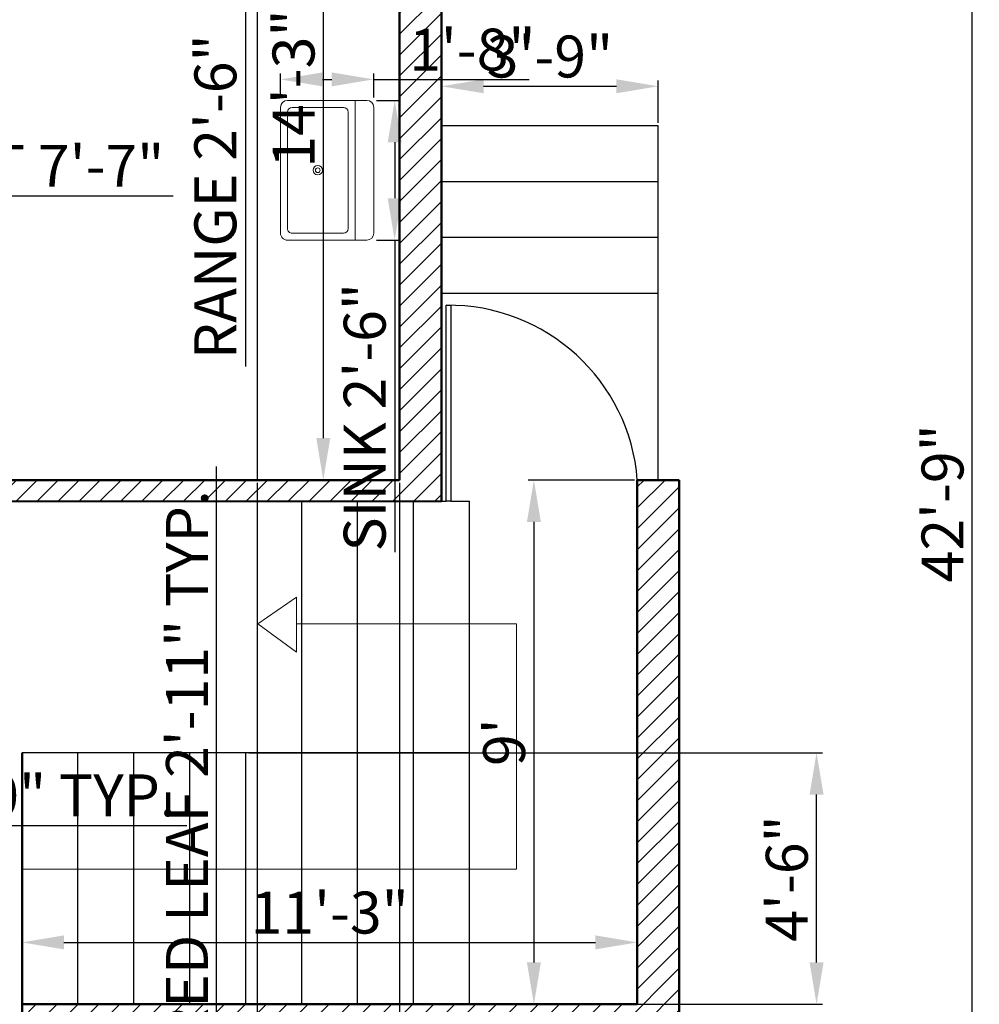
# Model space of a CAD drawing. Units: inches. Extents: x 5928 to 6612, y 5674 to 6320.
# Tile 4 of 5: x 6407 to 6612, y 5862 to 6074. Entities that reach past the tile are written whole.
import ezdxf

# ---------------------------------------------------------------- set-up
doc = ezdxf.new("R2010")
doc.units = ezdxf.units.IN
for name, color, linetype, lineweight in [('A-ANNO-DIMS', 2, 'Continuous', 18), ('A-ANNO-SYMB', 2, 'Continuous', 18), ('A-DOOR', 3, 'Continuous', 25), ('A-FLOR-CASE', 8, 'Continuous', 25), ('A-FLOR-FIXT', 9, 'Continuous', 18), ('A-FLOR-STRS', 7, 'Continuous', 25), ('A-WALL', 7, 'Continuous', 50), ('A-WALL-PATT', 252, 'Continuous', 13)]:
    doc.layers.add(name, color=color, linetype=linetype, lineweight=lineweight)
doc.styles.get("Standard").update_dxf_attribs({"font": 'arial.ttf'})
doc.dimstyles.new('ISO-25', dxfattribs={"dimtxt": 9, "dimasz": 9, "dimexe": 1.25, "dimexo": 0.625, "dimtad": 1, "dimdec": 1, "dimrnd": 9, "dimlunit": 3, "dimtxsty": 'Standard', "dimcen": 2.5, "dimadec": 0, "dimazin": 0, "dimtfac": 1, "dimtdec": 1, "dimtmove": 0, "dimatfit": 3, "dimfxl": 1, "dimarcsym": 0})

# ---------------------------------------------------------------- blocks, each defined once
blk = doc.blocks.new('*D1')
at = {"layer": 'A-ANNO-DIMS', "color": 0, "lineweight": -2, "transparency": 16777216}
for p, q in [((6497.03, 6051.41), (6497.03, 6060.5)), ((6543.53, 6051.41), (6543.53, 6060.5)), ((6506.03, 6059.25), (6534.53, 6059.25))]:
    blk.add_line(p, q, dxfattribs=at)
at = {"layer": 'A-ANNO-DIMS', "color": 0, "transparency": 16777216}
for points in [[(6506.03, 6060.75), (6506.03, 6057.75), (6497.03, 6059.25)], [(6534.53, 6060.75), (6534.53, 6057.75), (6543.53, 6059.25)]]:
    blk.add_solid(points, dxfattribs=at)
at = {"layer": 'Defpoints', "color": 0, "transparency": 16777216}
for p in [(6543.53, 6059.25), (6497.03, 6050.78), (6543.53, 6050.78)]:
    blk.add_point(p, dxfattribs=at)
at = {"layer": 'A-ANNO-DIMS', "color": 0, "transparency": 16777216, "insert": (6520.28, 6064.47), "char_height": 9, "attachment_point": 5}
blk.add_mtext('3\'-9"', dxfattribs=at)
blk = doc.blocks.new('Sink-single - 30 in top')
blk.add_line((-15, -3.999996), (15, -3.999996))
for points in [[(-13.5, 0), (13.5, 0)], [(-15, -18.499996), (-15, -1.5)], [(15, -1.5), (15, -18.499996)], [(-12.5, -5.499996), (12.5, -5.499996)], [(-13.5, -17.499996), (-13.5, -6.499996)], [(13.5, -6.499996), (13.5, -17.499996)], [(12.5, -18.499996), (-12.5, -18.499996)], [(13.5, -19.999996), (-13.5, -19.999996)]]:
    blk.add_lwpolyline(points)
for radius in [1, 0.5]:
    blk.add_circle((0, -11.999996), radius)
for centre, radius, start, end in [((-13.5, -1.5), 1.5, 90, 180), ((13.5, -1.5), 1.5, 0, 90), ((-12.5, -6.499996), 1, 90, 180), ((12.5, -6.499996), 1, 0, 90), ((-13.5, -18.499996), 1.5, 180, 270), ((-12.5, -17.499996), 1, 180, 270), ((12.5, -17.499996), 1, 270, 0), ((13.5, -18.499996), 1.5, 270, 0)]:
    blk.add_arc(centre, radius, start, end)
blk = doc.blocks.new('*D32')
at = {"layer": 'A-ANNO-DIMS', "color": 0, "lineweight": -2, "transparency": 16777216}
for p, q in [((6538.4, 5974.76), (6515.59, 5974.76)), ((6516.84, 5965.76), (6516.84, 5871.26)), ((6538.4, 5862.26), (6515.59, 5862.26))]:
    blk.add_line(p, q, dxfattribs=at)
at = {"layer": 'A-ANNO-DIMS', "color": 0, "transparency": 16777216}
for points in [[(6515.34, 5965.76), (6518.34, 5965.76), (6516.84, 5974.76)], [(6515.34, 5871.26), (6518.34, 5871.26), (6516.84, 5862.26)]]:
    blk.add_solid(points, dxfattribs=at)
at = {"layer": 'Defpoints', "color": 0, "transparency": 16777216}
for p in [(6539.03, 5974.76), (6516.84, 5862.26), (6539.03, 5862.26)]:
    blk.add_point(p, dxfattribs=at)
at = {"layer": 'A-ANNO-DIMS', "color": 0, "transparency": 16777216, "insert": (6511.62, 5918.51), "char_height": 9, "attachment_point": 5, "rotation": 90}
blk.add_mtext("9'", dxfattribs=at)
blk = doc.blocks.new('*D33')
at = {"layer": 'A-ANNO-DIMS', "color": 0, "lineweight": -2, "transparency": 16777216}
for p, q in [((6407.03, 5862.89), (6407.03, 5876.8)), ((6539.03, 5862.89), (6539.03, 5876.8)), ((6416.03, 5875.55), (6530.03, 5875.55))]:
    blk.add_line(p, q, dxfattribs=at)
at = {"layer": 'A-ANNO-DIMS', "color": 0, "transparency": 16777216}
for points in [[(6416.03, 5877.05), (6416.03, 5874.05), (6407.03, 5875.55)], [(6530.03, 5877.05), (6530.03, 5874.05), (6539.03, 5875.55)]]:
    blk.add_solid(points, dxfattribs=at)
at = {"layer": 'Defpoints', "color": 0, "transparency": 16777216}
for p in [(6539.03, 5875.55), (6407.03, 5862.26), (6539.03, 5862.26)]:
    blk.add_point(p, dxfattribs=at)
at = {"layer": 'A-ANNO-DIMS', "color": 0, "transparency": 16777216, "insert": (6473.03, 5880.78), "char_height": 9, "attachment_point": 5}
blk.add_mtext('11\'-3"', dxfattribs=at)
blk = doc.blocks.new('*D34')
at = {"layer": 'A-ANNO-DIMS', "color": 0, "lineweight": -2, "transparency": 16777216}
for p, q in [((6487.4, 6142.76), (6470.41, 6142.76)), ((6471.66, 6133.76), (6471.66, 5983.76)), ((6487.4, 5974.76), (6470.41, 5974.76))]:
    blk.add_line(p, q, dxfattribs=at)
at = {"layer": 'A-ANNO-DIMS', "color": 0, "transparency": 16777216}
for points in [[(6470.16, 6133.76), (6473.16, 6133.76), (6471.66, 6142.76)], [(6470.16, 5983.76), (6473.16, 5983.76), (6471.66, 5974.76)]]:
    blk.add_solid(points, dxfattribs=at)
at = {"layer": 'Defpoints', "color": 0, "transparency": 16777216}
for p in [(6488.03, 6142.76), (6471.66, 5974.76), (6488.03, 5974.76)]:
    blk.add_point(p, dxfattribs=at)
at = {"layer": 'A-ANNO-DIMS', "color": 0, "transparency": 16777216, "insert": (6466.44, 6058.76), "char_height": 9, "attachment_point": 5, "rotation": 90}
blk.add_mtext('14\'-3"', dxfattribs=at)
blk = doc.blocks.new('*D37')
at = {"layer": 'A-ANNO-DIMS', "color": 0, "lineweight": -2, "transparency": 16777216}
for p, q in [((6497.65, 6228.26), (6612.14, 6228.26)), ((6610.89, 5720.26), (6610.89, 6219.26)), ((6424.38, 5711.26), (6612.14, 5711.26))]:
    blk.add_line(p, q, dxfattribs=at)
at = {"layer": 'A-ANNO-DIMS', "color": 0, "transparency": 16777216}
for points in [[(6609.39, 6219.26), (6612.39, 6219.26), (6610.89, 6228.26)], [(6609.39, 5720.26), (6612.39, 5720.26), (6610.89, 5711.26)]]:
    blk.add_solid(points, dxfattribs=at)
at = {"layer": 'Defpoints', "color": 0, "transparency": 16777216}
for p in [(6497.03, 6228.26), (6610.89, 6228.26), (6423.76, 5711.26)]:
    blk.add_point(p, dxfattribs=at)
at = {"layer": 'A-ANNO-DIMS', "color": 0, "transparency": 16777216, "insert": (6605.67, 5969.76), "char_height": 9, "attachment_point": 5, "rotation": 90}
blk.add_mtext('42\'-9"', dxfattribs=at)
blk = doc.blocks.new('DOOR-LEAF-42IN')
for p, q in [((0, 0), (0, 42)), ((0, 42), (1, 42)), ((1, 42), (1, 0)), ((-1, 0), (0, 0)), ((1, 0), (0, 0))]:
    blk.add_line(p, q)
blk = doc.blocks.new('*D56')
at = {"layer": 'A-ANNO-DIMS', "color": 0, "lineweight": -2, "transparency": 16777216}
for p, q in [((6280.02, 5909.02), (6280.02, 5899.4)), ((6340.02, 5909.02), (6340.02, 5899.4)), ((6289.02, 5900.65), (6331.02, 5900.65)), ((6340.02, 5900.65), (6442.41, 5900.65))]:
    blk.add_line(p, q, dxfattribs=at)
at = {"layer": 'A-ANNO-DIMS', "color": 0, "transparency": 16777216}
for points in [[(6289.02, 5902.15), (6289.02, 5899.15), (6280.02, 5900.65)], [(6331.02, 5902.15), (6331.02, 5899.15), (6340.02, 5900.65)]]:
    blk.add_solid(points, dxfattribs=at)
at = {"layer": 'Defpoints', "color": 0, "transparency": 16777216}
for p in [(6280.02, 5909.65), (6340.02, 5909.65), (6340.02, 5900.65)]:
    blk.add_point(p, dxfattribs=at)
at = {"layer": 'A-ANNO-DIMS', "color": 0, "transparency": 16777216, "insert": (6395.71, 5905.93), "char_height": 9, "attachment_point": 5}
blk.add_mtext('DESK 5\'-0" TYP.', dxfattribs=at)
blk = doc.blocks.new('*D62')
at = {"layer": 'A-ANNO-DIMS', "color": 0, "lineweight": -2, "transparency": 16777216}
for p, q in [((6448.73, 5820.79), (6448.73, 5977.68)), ((6444.07, 5820.79), (6449.98, 5820.79)), ((6448.73, 5794.57), (6448.73, 5811.79)), ((6444.07, 5785.57), (6449.98, 5785.57))]:
    blk.add_line(p, q, dxfattribs=at)
at = {"layer": 'A-ANNO-DIMS', "color": 0, "transparency": 16777216}
for points in [[(6447.23, 5811.79), (6450.23, 5811.79), (6448.73, 5820.79)], [(6447.23, 5794.57), (6450.23, 5794.57), (6448.73, 5785.57)]]:
    blk.add_solid(points, dxfattribs=at)
at = {"layer": 'Defpoints', "color": 0, "transparency": 16777216}
for p in [(6443.45, 5820.79), (6448.73, 5820.79), (6443.45, 5785.57)]:
    blk.add_point(p, dxfattribs=at)
at = {"layer": 'A-ANNO-DIMS', "color": 0, "transparency": 16777216, "insert": (6443.58, 5903.73), "char_height": 9, "attachment_point": 5, "rotation": 90}
blk.add_mtext('PAIRED LEAF 2\'-11" TYP.', dxfattribs=at)
blk = doc.blocks.new('*D64')
at = {"layer": 'A-ANNO-DIMS', "color": 0, "lineweight": -2, "transparency": 16777216}
for p, q in [((6239.27, 6048.77), (6239.27, 6034.49)), ((6330.27, 6048.77), (6330.27, 6034.49)), ((6248.27, 6035.74), (6321.27, 6035.74)), ((6330.27, 6035.74), (6439.44, 6035.74))]:
    blk.add_line(p, q, dxfattribs=at)
at = {"layer": 'A-ANNO-DIMS', "color": 0, "transparency": 16777216}
for points in [[(6248.27, 6037.24), (6248.27, 6034.24), (6239.27, 6035.74)], [(6321.27, 6037.24), (6321.27, 6034.24), (6330.27, 6035.74)]]:
    blk.add_solid(points, dxfattribs=at)
at = {"layer": 'Defpoints', "color": 0, "transparency": 16777216}
for p in [(6239.27, 6049.39), (6330.27, 6049.39), (6330.27, 6035.74)]:
    blk.add_point(p, dxfattribs=at)
at = {"layer": 'A-ANNO-DIMS', "color": 0, "transparency": 16777216, "insert": (6389.36, 6041.02), "char_height": 9, "attachment_point": 5}
blk.add_mtext('DINING SET 7\'-7"', dxfattribs=at)
blk = doc.blocks.new('*D66')
at = {"layer": 'A-ANNO-DIMS', "color": 0, "lineweight": -2, "transparency": 16777216}
for p, q in [((6458.82, 6111), (6453.69, 6111)), ((6454.94, 6102), (6454.94, 6090)), ((6458.82, 6081), (6453.69, 6081)), ((6454.94, 6081), (6454.94, 5999.09))]:
    blk.add_line(p, q, dxfattribs=at)
at = {"layer": 'A-ANNO-DIMS', "color": 0, "transparency": 16777216}
for points in [[(6453.44, 6102), (6456.44, 6102), (6454.94, 6111)], [(6453.44, 6090), (6456.44, 6090), (6454.94, 6081)]]:
    blk.add_solid(points, dxfattribs=at)
at = {"layer": 'Defpoints', "color": 0, "transparency": 16777216}
for p in [(6459.44, 6111), (6454.94, 6081), (6459.44, 6081)]:
    blk.add_point(p, dxfattribs=at)
at = {"layer": 'A-ANNO-DIMS', "color": 0, "transparency": 16777216, "insert": (6449.67, 6035.54), "char_height": 9, "attachment_point": 5, "rotation": 90}
blk.add_mtext('RANGE 2\'-6"', dxfattribs=at)
blk = doc.blocks.new('*D68')
at = {"layer": 'A-ANNO-DIMS', "color": 0, "lineweight": -2, "transparency": 16777216}
for p, q in [((6483.1, 6056.23), (6488.23, 6056.23)), ((6486.98, 6047.23), (6486.98, 6035.23)), ((6483.1, 6026.23), (6488.23, 6026.23)), ((6486.98, 6026.23), (6486.98, 5959.26))]:
    blk.add_line(p, q, dxfattribs=at)
at = {"layer": 'A-ANNO-DIMS', "color": 0, "transparency": 16777216}
for points in [[(6485.48, 6047.23), (6488.48, 6047.23), (6486.98, 6056.23)], [(6485.48, 6035.23), (6488.48, 6035.23), (6486.98, 6026.23)]]:
    blk.add_solid(points, dxfattribs=at)
at = {"layer": 'Defpoints', "color": 0, "transparency": 16777216}
for p in [(6482.48, 6056.23), (6482.48, 6026.23), (6486.98, 6026.23)]:
    blk.add_point(p, dxfattribs=at)
at = {"layer": 'A-ANNO-DIMS', "color": 0, "transparency": 16777216, "insert": (6481.7, 5988.24), "char_height": 9, "attachment_point": 5, "rotation": 90}
blk.add_mtext('SINK 2\'-6"', dxfattribs=at)
blk = doc.blocks.new('*D69')
at = {"layer": 'A-ANNO-DIMS', "color": 0, "lineweight": -2, "transparency": 16777216}
for p, q in [((6462.48, 6056.85), (6462.48, 6061.98)), ((6482.48, 6056.85), (6482.48, 6061.98)), ((6471.48, 6060.73), (6473.48, 6060.73)), ((6482.48, 6060.73), (6515.81, 6060.73))]:
    blk.add_line(p, q, dxfattribs=at)
at = {"layer": 'A-ANNO-DIMS', "color": 0, "transparency": 16777216}
for points in [[(6471.48, 6062.23), (6471.48, 6059.23), (6462.48, 6060.73)], [(6473.48, 6062.23), (6473.48, 6059.23), (6482.48, 6060.73)]]:
    blk.add_solid(points, dxfattribs=at)
at = {"layer": 'Defpoints', "color": 0, "transparency": 16777216}
for p in [(6482.48, 6060.73), (6462.48, 6056.23), (6482.48, 6056.23)]:
    blk.add_point(p, dxfattribs=at)
at = {"layer": 'A-ANNO-DIMS', "color": 0, "transparency": 16777216, "insert": (6503.64, 6065.95), "char_height": 9, "attachment_point": 5}
blk.add_mtext('1\'-8"', dxfattribs=at)
blk = doc.blocks.new('*D77')
at = {"layer": 'A-ANNO-DIMS', "color": 0, "lineweight": -2, "transparency": 16777216}
for p, q in [((6457.49, 5974.14), (6457.49, 5680.56)), ((6488.03, 5974.14), (6488.03, 5680.56)), ((6466.49, 5681.81), (6479.03, 5681.81)), ((6488.03, 5681.81), (6543.33, 5681.81))]:
    blk.add_line(p, q, dxfattribs=at)
at = {"layer": 'A-ANNO-DIMS', "color": 0, "transparency": 16777216}
for points in [[(6466.49, 5683.31), (6466.49, 5680.31), (6457.49, 5681.81)], [(6479.03, 5683.31), (6479.03, 5680.31), (6488.03, 5681.81)]]:
    blk.add_solid(points, dxfattribs=at)
at = {"layer": 'Defpoints', "color": 0, "transparency": 16777216}
for p in [(6457.49, 5974.76), (6488.03, 5974.76), (6488.03, 5681.81)]:
    blk.add_point(p, dxfattribs=at)
at = {"layer": 'A-ANNO-DIMS', "color": 0, "transparency": 16777216, "insert": (6520.18, 5687.09), "char_height": 9, "attachment_point": 5}
blk.add_mtext('2\'-6 1/2"', dxfattribs=at)
blk = doc.blocks.new('*D78')
at = {"layer": 'A-ANNO-DIMS', "color": 0, "lineweight": -2, "transparency": 16777216}
for p, q in [((6455.65, 5916.26), (6578.73, 5916.26)), ((6577.48, 5871.26), (6577.48, 5907.26)), ((6455.65, 5862.26), (6578.73, 5862.26))]:
    blk.add_line(p, q, dxfattribs=at)
at = {"layer": 'A-ANNO-DIMS', "color": 0, "transparency": 16777216}
for points in [[(6575.98, 5907.26), (6578.98, 5907.26), (6577.48, 5916.26)], [(6575.98, 5871.26), (6578.98, 5871.26), (6577.48, 5862.26)]]:
    blk.add_solid(points, dxfattribs=at)
at = {"layer": 'Defpoints', "color": 0, "transparency": 16777216}
for p in [(6455.03, 5916.26), (6577.48, 5916.26), (6455.03, 5862.26)]:
    blk.add_point(p, dxfattribs=at)
at = {"layer": 'A-ANNO-DIMS', "color": 0, "transparency": 16777216, "insert": (6572.26, 5889.26), "char_height": 9, "attachment_point": 5, "rotation": 90}
blk.add_mtext('4\'-6"', dxfattribs=at)

msp = doc.modelspace()

# ---------------------------------------------------------------- hatches: boundary and pattern name
at = {"layer": 'A-WALL-PATT'}
h = msp.add_hatch(dxfattribs=at)
h.set_pattern_fill('ANSI31', color=256)
h.paths.add_polyline_path([(6071.03, 6165.76), (6215.03, 6165.76), (6215.03, 5969.77), (6215.03, 5950.32), (6219.53, 5950.32), (6219.53, 6142.76), (6239.11, 6142.76), (6239.11, 6151.76), (6224.03, 6151.76), (6224.03, 6174.76), (6062.03, 6174.76), (6062.03, 5969.76), (6062.03, 5894.26), (6108.76, 5894.26), (6108.76, 5711.26), (6423.76, 5711.26), (6423.76, 5750.35), (6414.76, 5750.35), (6414.76, 5720.26), (6266.26, 5720.26), (6266.26, 5862.26), (6361.1, 5862.26), (6361.1, 5866.76), (6261.76, 5866.76), (6261.76, 5720.26), (6117.76, 5720.26), (6117.76, 5792.26), (6218.26, 5792.26), (6218.26, 5796.76), (6117.76, 5796.76), (6117.76, 5898.76), (6213.76, 5898.76), (6213.76, 5828.21, -0.018207), (6216.01, 5828.09), (6218.26, 5828.09), (6218.26, 5903.26), (6117.76, 5903.26), (6071.03, 5903.26), (6071.03, 5969.77), (6071.03, 6041.26), (6117.76, 6041.26), (6172.44, 6041.26), (6172.44, 6045.76), (6117.76, 6045.76), (6071.03, 6045.76)])
h.paths.add_polyline_path([(6368.03, 6219.26), (6488.03, 6219.26), (6488.03, 6147.26), (6403.79, 6147.26), (6403.79, 6142.76), (6488.03, 6142.76), (6488.03, 5974.76), (6363.53, 5974.76), (6363.53, 5970.11), (6497.03, 5970.26), (6497.03, 6142.76), (6497.03, 6228.26), (6359.03, 6228.26), (6359.03, 6151.76), (6344.11, 6151.76), (6344.11, 6142.76), (6363.53, 6142.76), (6363.53, 6013.35), (6368.03, 6013.35), (6368.03, 6142.76)])
h.paths.add_polyline_path([(6344.11, 6196.21, 0.265753), (6295.16, 6228.26), (6288.06, 6228.26, 0.265753), (6239.11, 6196.21), (6239.11, 6142.76), (6243.61, 6142.76), (6243.61, 6196.76), (6243.45, 6196.76, -0.514089), (6339.79, 6196.74), (6339.61, 6196.76), (6339.61, 6142.76), (6344.11, 6142.76)])
h.paths.add_polyline_path([(6339.61, 6147.26), (6327.61, 6147.26), (6327.61, 6142.76), (6339.61, 6142.76)], flags=17)
h.paths.add_polyline_path([(6255.61, 6147.26), (6243.61, 6147.26), (6243.61, 6142.76), (6255.61, 6142.76)], flags=17)
h.paths.add_polyline_path([(6548.03, 5974.76), (6539.03, 5974.76), (6539.03, 5862.26), (6407.03, 5862.26), (6407.03, 5853.26), (6414.76, 5853.26), (6414.76, 5820.79), (6423.76, 5820.79), (6423.76, 5853.26), (6548.03, 5853.26)])

# ---------------------------------------------------------------- linework, layer by layer
at = {"layer": 'A-ANNO-SYMB'}
for p, q in [((6457.59, 5943.9), (6465.93, 5949.64)), ((6465.93, 5949.64), (6465.93, 5937.81)), ((6465.93, 5937.81), (6457.59, 5943.9)), ((6513.09, 5943.9), (6465.93, 5943.9)), ((6513.09, 5891.29), (6513.09, 5943.9)), ((6407.03, 5891.29), (6407.03, 5891.29)), ((6407.03, 5891.29), (6513.09, 5891.29))]:
    msp.add_line(p, q, dxfattribs=at)
at = {"layer": 'A-DOOR'}
msp.add_arc((6498.53, 5971.65), 40.62, 4.4005, 90.7053, dxfattribs=at)
at = {"layer": 'A-FLOR-CASE'}
msp.add_line((6457.49, 6142.76), (6457.49, 5974.76), dxfattribs=at)
at = {"layer": 'A-FLOR-STRS'}
for p, q in [((6543.53, 6050.78), (6497.03, 6050.78)), ((6543.53, 5974.76), (6543.53, 6050.78)), ((6543.53, 6038.78), (6497.03, 6038.78)), ((6543.53, 6026.78), (6497.03, 6026.78)), ((6543.53, 6014.78), (6497.03, 6014.78)), ((6419.03, 5970.17), (6419.03, 5970.26)), ((6431.03, 5970.19), (6431.03, 5970.26)), ((6443.03, 5970.2), (6443.03, 5970.26)), ((6455.03, 5970.22), (6455.03, 5970.26)), ((6467.03, 5862.26), (6467.03, 5970.26)), ((6479.03, 5862.26), (6479.03, 5970.26)), ((6491.03, 5862.26), (6491.03, 5970.26)), ((6499.03, 5970.26), (6503.03, 5970.26)), ((6503.03, 5862.26), (6503.03, 5970.26)), ((6503.03, 5916.26), (6407.03, 5916.26)), ((6419.03, 5862.26), (6419.03, 5916.26)), ((6431.03, 5862.26), (6431.03, 5916.26)), ((6443.03, 5862.26), (6443.03, 5916.26)), ((6455.03, 5862.26), (6455.03, 5916.26))]:
    msp.add_line(p, q, dxfattribs=at)
at = {"layer": 'A-WALL'}
for p, q in [((6488.03, 5974.76), (6488.03, 6142.76)), ((6497.03, 5970.26), (6497.03, 6142.76)), ((6488.03, 5974.76), (6363.53, 5974.76)), ((6548.03, 5974.76), (6539.03, 5974.76)), ((6539.03, 5862.26), (6539.03, 5974.76)), ((6548.03, 5853.26), (6548.03, 5974.76)), ((6497.03, 5970.26), (6363.53, 5970.11)), ((6407.03, 5853.26), (6407.03, 5916.26)), ((6539.03, 5862.26), (6407.03, 5862.26))]:
    msp.add_line(p, q, dxfattribs=at)

# ---------------------------------------------------------------- block references
at = {"layer": 'A-DOOR'}
msp.add_blockref('DOOR-LEAF-42IN', (6498.03, 5970.26), dxfattribs=at)
at = {"layer": 'A-FLOR-FIXT', "rotation": 270}
msp.add_blockref('Sink-single - 30 in top', (6482.48, 6041.23), dxfattribs=at)

# ---------------------------------------------------------------- dimensions: what is measured, and where the dimension line sits
at = {"layer": 'A-ANNO-DIMS'}
for base, p1, p2, override, picture, middle in [((6610.89, 6228.26), (6423.76, 5711.26), (6497.03, 6228.26), {"dimclrd": 0, "dimclre": 0, "dimclrt": 0}, '*D37', (6605.67, 5969.76)), ((6471.66, 5974.76), (6488.03, 6142.76), (6488.03, 5974.76), {"dimclrd": 0, "dimclre": 0, "dimclrt": 0}, '*D34', (6466.44, 6058.76)), ((6516.84, 5862.26), (6539.03, 5974.76), (6539.03, 5862.26), {"dimclrd": 0, "dimclre": 0, "dimclrt": 0}, '*D32', (6511.62, 5918.51)), ((6577.48, 5916.26), (6455.03, 5862.26), (6455.03, 5916.26), {"dimdec": 1, "dimlfac": 1, "dimrnd": 0, "dimzin": 1, "dimdsep": 46, "dimlunit": 4, "dimfrac": 2}, '*D78', (6572.26, 5889.26))]:
    dim = msp.add_linear_dim(base=base, p1=p1, p2=p2, angle=90, dimstyle='ISO-25', override=override, dxfattribs=at)
    dim.commit()
    dim.dimension.update_dxf_attribs({"geometry": picture, "text_midpoint": middle})
for base, p1, p2, angle, text, picture, middle in [((6454.94, 6081), (6459.44, 6111), (6459.44, 6081), 270, 'RANGE <>', '*D66', (6449.67, 6035.54)), ((6486.98, 6026.23), (6482.48, 6056.23), (6482.48, 6026.23), 270, 'SINK <>', '*D68', (6481.7, 5988.24)), ((6448.73, 5820.79), (6443.45, 5785.57), (6443.45, 5820.79), 90, 'PAIRED LEAF <> TYP.', '*D62', (6443.58, 5903.73))]:
    dim = msp.add_linear_dim(base=base, p1=p1, p2=p2, angle=angle, text=text, dimstyle='ISO-25', override={"dimdec": 1, "dimlfac": 1, "dimrnd": 0, "dimzin": 1, "dimdsep": 46, "dimlunit": 4, "dimfrac": 2}, dxfattribs=at)
    dim.commit()
    dim.dimension.update_dxf_attribs({"geometry": picture, "text_midpoint": middle})
for base, p1, p2, override, picture, middle in [((6482.48, 6060.73), (6462.48, 6056.23), (6482.48, 6056.23), {"dimdec": 1, "dimlfac": 1, "dimrnd": 0, "dimzin": 1, "dimdsep": 46, "dimlunit": 4, "dimfrac": 2}, '*D69', (6503.64, 6065.95)), ((6543.53, 6059.25), (6497.03, 6050.78), (6543.53, 6050.78), {"dimclrd": 0, "dimclre": 0, "dimclrt": 0}, '*D1', (6520.28, 6064.47)), ((6488.03, 5681.81), (6457.49, 5974.76), (6488.03, 5974.76), {"dimdec": 1, "dimlfac": 1, "dimrnd": 0, "dimzin": 1, "dimdsep": 46, "dimlunit": 4, "dimfrac": 2}, '*D77', (6520.18, 5687.09)), ((6539.03, 5875.55), (6407.03, 5862.26), (6539.03, 5862.26), {"dimclrd": 0, "dimclre": 0, "dimclrt": 0}, '*D33', (6473.03, 5880.78))]:
    dim = msp.add_linear_dim(base=base, p1=p1, p2=p2, dimstyle='ISO-25', override=override, dxfattribs=at)
    dim.commit()
    dim.dimension.update_dxf_attribs({"geometry": picture, "text_midpoint": middle})
for base, p1, p2, text, picture, middle in [((6330.27, 6035.74), (6239.27, 6049.39), (6330.27, 6049.39), 'DINING SET <>', '*D64', (6389.36, 6041.02)), ((6340.02, 5900.65), (6280.02, 5909.65), (6340.02, 5909.65), 'DESK <> TYP.', '*D56', (6395.71, 5905.93))]:
    dim = msp.add_linear_dim(base=base, p1=p1, p2=p2, text=text, dimstyle='ISO-25', override={"dimdec": 1, "dimlfac": 1, "dimrnd": 0, "dimzin": 1, "dimdsep": 46, "dimlunit": 4, "dimfrac": 2}, dxfattribs=at)
    dim.commit()
    dim.dimension.update_dxf_attribs({"geometry": picture, "text_midpoint": middle})

doc.saveas('drawing.dxf')
